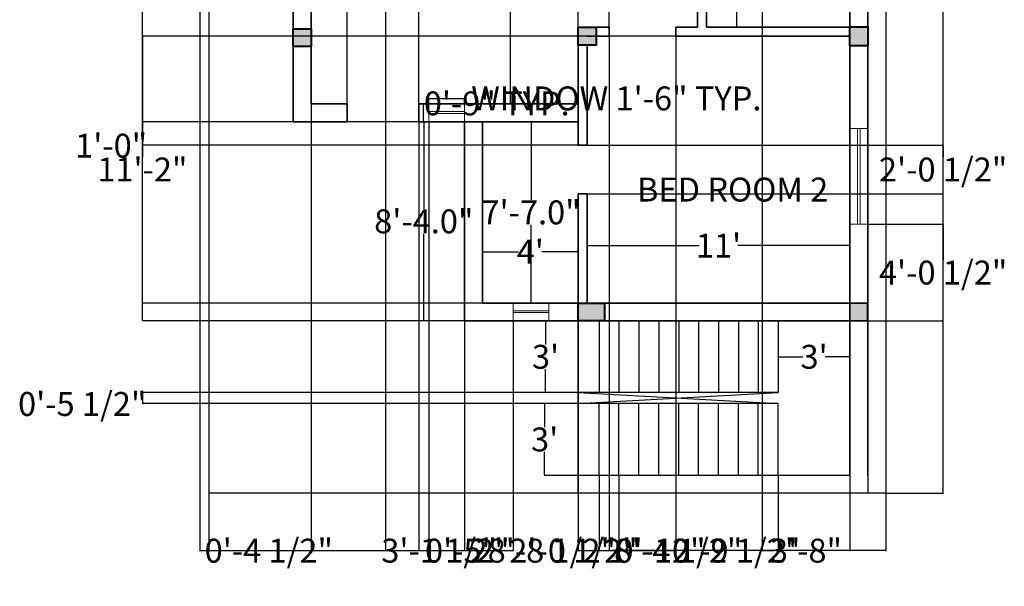
# Model space of a CAD drawing. Units: inches. Extents: x -132 to 363, y -548 to 79.
# Tile 1 of 3: x -132 to 363, y -548 to -264. Entities that reach past the tile are written whole.
import ezdxf

# ---------------------------------------------------------------- set-up
doc = ezdxf.new("R2010")
doc.units = ezdxf.units.IN
doc.header["$MEASUREMENT"] = 0
for name, color, linetype, lineweight in [('A-ANNO-DIMS', 2, 'Continuous', 18), ('A-AREA-IDEN', 7, 'Continuous', 25), ('A-COLS', 7, 'Continuous', 40), ('A-COLS-PATT', 252, 'Continuous', 13), ('A-FLOR-STRS', 3, 'Continuous', 25), ('A-GLAZ', 4, 'Continuous', 18), ('A-WALL', 7, 'Continuous', 35), ('C-PROP', 8, 'Continuous', 25)]:
    doc.layers.add(name, color=color, linetype=linetype, lineweight=lineweight)
doc.styles.get("Standard").update_dxf_attribs({"font": 'arial.ttf'})
doc.dimstyles.get("Standard").update_dxf_attribs({"dimtxt": 12, "dimasz": 0.18, "dimexe": 0.18, "dimexo": 0.0625, "dimgap": 0.09, "dimtad": 0, "dimtih": 1, "dimtoh": 1, "dimdec": 1, "dimzin": 0, "dimdsep": 46, "dimlunit": 3, "dimtxsty": 'Standard', "dimcen": 0.09, "dimadec": 0, "dimazin": 0, "dimtfac": 1, "dimtdec": 1, "dimtofl": 0, "dimtmove": 0, "dimatfit": 3, "dimfxl": 1, "dimtolj": 1, "dimtzin": 0, "dimarcsym": 0})

# ---------------------------------------------------------------- blocks, each defined once
blk = doc.blocks.new('*D6')
at = {"layer": 'A-ANNO-DIMS', "color": 0, "lineweight": -2, "transparency": 16777216}
for p, q in [((213.08, -219.61), (228.48, -219.61)), ((228.3, -219.79), (228.3, -237.52)), ((228.3, -267.43), (228.3, -249.7)), ((213.08, -267.61), (228.48, -267.61))]:
    blk.add_line(p, q, dxfattribs=at)
at = {"layer": 'A-ANNO-DIMS', "color": 0, "transparency": 16777216}
for points in [[(228.27, -219.79), (228.33, -219.79), (228.3, -219.61)], [(228.27, -267.43), (228.33, -267.43), (228.3, -267.61)]]:
    blk.add_solid(points, dxfattribs=at)
at = {"layer": 'Defpoints', "color": 0, "transparency": 16777216}
for p in [(213.02, -219.61), (213.02, -267.61), (228.3, -267.61)]:
    blk.add_point(p, dxfattribs=at)
at = {"layer": 'A-ANNO-DIMS', "color": 0, "transparency": 16777216, "insert": (228.3, -243.61), "char_height": 12, "attachment_point": 5}
blk.add_mtext("\\A1;4'", dxfattribs=at)
blk = doc.blocks.new('*D8')
at = {"layer": 'A-ANNO-DIMS', "color": 0, "lineweight": -2, "transparency": 16777216}
for p, q in [((153.02, -378.62), (153.02, -377.14)), ((153.2, -377.32), (209.31, -377.32)), ((284.84, -377.32), (228.72, -377.32)), ((285.02, -378.62), (285.02, -377.14))]:
    blk.add_line(p, q, dxfattribs=at)
at = {"layer": 'A-ANNO-DIMS', "color": 0, "transparency": 16777216}
for points in [[(153.2, -377.29), (153.2, -377.35), (153.02, -377.32)], [(284.84, -377.29), (284.84, -377.35), (285.02, -377.32)]]:
    blk.add_solid(points, dxfattribs=at)
at = {"layer": 'Defpoints', "color": 0, "transparency": 16777216}
for p in [(153.02, -378.68), (285.02, -377.32), (285.02, -378.68)]:
    blk.add_point(p, dxfattribs=at)
at = {"layer": 'A-ANNO-DIMS', "color": 0, "transparency": 16777216, "insert": (219.02, -377.32), "char_height": 12, "attachment_point": 5}
blk.add_mtext("\\A1;11'", dxfattribs=at)
blk = doc.blocks.new('*D9')
at = {"layer": 'A-ANNO-DIMS', "color": 0, "lineweight": -2, "transparency": 16777216}
for p, q in [((249.02, -433.05), (249.02, -432.93)), ((249.2, -433.11), (261.41, -433.11)), ((284.84, -433.11), (272.62, -433.11)), ((285.02, -433.05), (285.02, -432.93))]:
    blk.add_line(p, q, dxfattribs=at)
at = {"layer": 'A-ANNO-DIMS', "color": 0, "transparency": 16777216}
for points in [[(249.2, -433.08), (249.2, -433.14), (249.02, -433.11)], [(284.84, -433.08), (284.84, -433.14), (285.02, -433.11)]]:
    blk.add_solid(points, dxfattribs=at)
at = {"layer": 'Defpoints', "color": 0, "transparency": 16777216}
for p in [(249.02, -433.11), (285.02, -433.11), (285.02, -433.11)]:
    blk.add_point(p, dxfattribs=at)
at = {"layer": 'A-ANNO-DIMS', "color": 0, "transparency": 16777216, "insert": (267.02, -433.11), "char_height": 12, "attachment_point": 5}
blk.add_mtext("\\A1;3'", dxfattribs=at)
blk = doc.blocks.new('*D10')
at = {"layer": 'A-ANNO-DIMS', "color": 0, "lineweight": -2, "transparency": 16777216}
for p, q in [((148.45, -415.11), (132, -415.11)), ((132.18, -415.29), (132.18, -426.89)), ((132.18, -450.93), (132.18, -439.33)), ((148.45, -451.11), (132, -451.11))]:
    blk.add_line(p, q, dxfattribs=at)
at = {"layer": 'A-ANNO-DIMS', "color": 0, "transparency": 16777216}
for points in [[(132.15, -415.29), (132.21, -415.29), (132.18, -415.11)], [(132.15, -450.93), (132.21, -450.93), (132.18, -451.11)]]:
    blk.add_solid(points, dxfattribs=at)
at = {"layer": 'Defpoints', "color": 0, "transparency": 16777216}
for p in [(148.52, -415.11), (132.18, -451.11), (148.52, -451.11)]:
    blk.add_point(p, dxfattribs=at)
at = {"layer": 'A-ANNO-DIMS', "color": 0, "transparency": 16777216, "insert": (132.18, -433.11), "char_height": 12, "attachment_point": 5}
blk.add_mtext("\\A1;3'", dxfattribs=at)
blk = doc.blocks.new('*D11')
at = {"layer": 'A-ANNO-DIMS', "color": 0, "lineweight": -2, "transparency": 16777216}
for p, q in [((148.45, -456.61), (131.55, -456.61)), ((131.73, -456.79), (131.73, -468.39)), ((131.73, -492.43), (131.73, -480.83)), ((148.45, -492.61), (131.55, -492.61))]:
    blk.add_line(p, q, dxfattribs=at)
at = {"layer": 'A-ANNO-DIMS', "color": 0, "transparency": 16777216}
for points in [[(131.7, -456.79), (131.76, -456.79), (131.73, -456.61)], [(131.7, -492.43), (131.76, -492.43), (131.73, -492.61)]]:
    blk.add_solid(points, dxfattribs=at)
at = {"layer": 'Defpoints', "color": 0, "transparency": 16777216}
for p in [(148.52, -456.61), (131.73, -492.61), (148.52, -492.61)]:
    blk.add_point(p, dxfattribs=at)
at = {"layer": 'A-ANNO-DIMS', "color": 0, "transparency": 16777216, "insert": (131.73, -474.61), "char_height": 12, "attachment_point": 5}
blk.add_mtext("\\A1;3'", dxfattribs=at)
blk = doc.blocks.new('*D12')
at = {"layer": 'A-ANNO-DIMS', "color": 0, "lineweight": -2, "transparency": 16777216}
for p, q in [((100.52, -380.31), (100.52, -380.19)), ((100.7, -380.37), (118.66, -380.37)), ((148.34, -380.37), (130.37, -380.37)), ((148.52, -380.31), (148.52, -380.19))]:
    blk.add_line(p, q, dxfattribs=at)
at = {"layer": 'A-ANNO-DIMS', "color": 0, "transparency": 16777216}
for points in [[(100.7, -380.34), (100.7, -380.4), (100.52, -380.37)], [(148.34, -380.34), (148.34, -380.4), (148.52, -380.37)]]:
    blk.add_solid(points, dxfattribs=at)
at = {"layer": 'Defpoints', "color": 0, "transparency": 16777216}
for p in [(100.52, -380.37), (148.52, -380.37), (148.52, -380.37)]:
    blk.add_point(p, dxfattribs=at)
at = {"layer": 'A-ANNO-DIMS', "color": 0, "transparency": 16777216, "insert": (124.52, -380.37), "char_height": 12, "attachment_point": 5}
blk.add_mtext("\\A1;4'", dxfattribs=at)
blk = doc.blocks.new('*D13')
at = {"layer": 'A-ANNO-DIMS', "color": 0, "lineweight": -2, "transparency": 16777216}
for p, q in [((120.95, -315.11), (125.08, -315.11)), ((124.9, -315.29), (124.9, -354.39)), ((124.9, -405.93), (124.9, -366.82)), ((124.97, -406.11), (125.08, -406.11))]:
    blk.add_line(p, q, dxfattribs=at)
at = {"layer": 'A-ANNO-DIMS', "color": 0, "transparency": 16777216}
for points in [[(124.87, -315.29), (124.93, -315.29), (124.9, -315.11)], [(124.87, -405.93), (124.93, -405.93), (124.9, -406.11)]]:
    blk.add_solid(points, dxfattribs=at)
at = {"layer": 'Defpoints', "color": 0, "transparency": 16777216}
for p in [(120.89, -315.11), (124.9, -406.11), (124.9, -406.11)]:
    blk.add_point(p, dxfattribs=at)
at = {"layer": 'A-ANNO-DIMS', "color": 0, "transparency": 16777216, "insert": (124.9, -360.61), "char_height": 12, "attachment_point": 5}
blk.add_mtext('\\A1;7\'-7.0"', dxfattribs=at)
blk = doc.blocks.new('*D14')
at = {"layer": 'A-ANNO-DIMS', "color": 0, "lineweight": -2, "transparency": 16777216}
for p, q in [((91.45, -315.11), (70.85, -315.11)), ((71.03, -315.29), (71.03, -358.89)), ((71.03, -414.93), (71.03, -371.32)), ((91.45, -415.11), (70.85, -415.11))]:
    blk.add_line(p, q, dxfattribs=at)
at = {"layer": 'A-ANNO-DIMS', "color": 0, "transparency": 16777216}
for points in [[(71, -315.29), (71.06, -315.29), (71.03, -315.11)], [(71, -414.93), (71.06, -414.93), (71.03, -415.11)]]:
    blk.add_solid(points, dxfattribs=at)
at = {"layer": 'Defpoints', "color": 0, "transparency": 16777216}
for p in [(91.52, -315.11), (71.03, -415.11), (91.52, -415.11)]:
    blk.add_point(p, dxfattribs=at)
at = {"layer": 'A-ANNO-DIMS', "color": 0, "transparency": 16777216, "insert": (71.03, -365.11), "char_height": 12, "attachment_point": 5}
blk.add_mtext('\\A1;8\'-4.0"', dxfattribs=at)
blk = doc.blocks.new('*D16')
at = {"layer": 'A-ANNO-DIMS', "color": 0, "lineweight": -2, "transparency": 16777216}
for p, q in [((148.45, -92.11), (114.32, -92.11)), ((114.5, -92.29), (114.5, -192.89)), ((114.5, -305.93), (114.5, -205.32)), ((148.45, -306.11), (114.32, -306.11))]:
    blk.add_line(p, q, dxfattribs=at)
at = {"layer": 'A-ANNO-DIMS', "color": 0, "transparency": 16777216}
for points in [[(114.47, -92.29), (114.53, -92.29), (114.5, -92.11)], [(114.47, -305.93), (114.53, -305.93), (114.5, -306.11)]]:
    blk.add_solid(points, dxfattribs=at)
at = {"layer": 'Defpoints', "color": 0, "transparency": 16777216}
for p in [(148.52, -92.11), (114.5, -306.11), (148.52, -306.11)]:
    blk.add_point(p, dxfattribs=at)
at = {"layer": 'A-ANNO-DIMS', "color": 0, "transparency": 16777216, "insert": (114.5, -199.11), "char_height": 12, "attachment_point": 5}
blk.add_mtext('\\A1;17\'-10.0"', dxfattribs=at)
blk = doc.blocks.new('WIN-48IN')
for p, q in [((48, 9), (0, 9)), ((0, 9), (0, 0)), ((0, 5.12), (48, 5.12)), ((48, 5.12), (0, 5.12)), ((48, 0), (48, 9)), ((0, 3.8), (48, 3.8)), ((0, 0), (48, 0))]:
    blk.add_line(p, q)
blk = doc.blocks.new('WIN-18IN')
for p, q in [((18, 9), (0, 9)), ((0, 9), (0, 0)), ((0, 6), (0, 0)), ((18, 5.06), (0, 5.06)), ((18, 0), (18, 9)), ((18, 0), (18, 6)), ((18, 4.2), (0, 4.2)), ((0, 0), (18, 0)), ((0, 0), (18, 0)), ((0, 0), (18, 0))]:
    blk.add_line(p, q)
blk = doc.blocks.new('*D23')
at = {"layer": 'A-ANNO-DIMS', "color": 0, "lineweight": -2, "transparency": 16777216}
for p, q in [((73.52, -306.05), (73.52, -303.23)), ((73.7, -303.41), (91.34, -303.41)), ((91.52, -306.05), (91.52, -303.23)), ((91.52, -303.41), (91.7, -303.41))]:
    blk.add_line(p, q, dxfattribs=at)
at = {"layer": 'A-ANNO-DIMS', "color": 0, "transparency": 16777216}
for points in [[(73.7, -303.38), (73.7, -303.44), (73.52, -303.41)], [(91.34, -303.38), (91.34, -303.44), (91.52, -303.41)]]:
    blk.add_solid(points, dxfattribs=at)
at = {"layer": 'Defpoints', "color": 0, "transparency": 16777216}
for p in [(73.52, -306.11), (91.52, -303.41), (91.52, -306.11)]:
    blk.add_point(p, dxfattribs=at)
at = {"layer": 'A-ANNO-DIMS', "color": 0, "transparency": 16777216, "insert": (167.71, -303.41), "char_height": 12, "attachment_point": 5}
blk.add_mtext('\\A1;WINDOW 1\'-6" TYP.', dxfattribs=at)
blk = doc.blocks.new('*D24')
at = {"layer": 'A-ANNO-DIMS', "color": 0, "lineweight": -2, "transparency": 16777216}
for p, q in [((73.45, -306.11), (70.64, -306.11)), ((70.82, -306.11), (70.82, -305.93)), ((70.82, -305.93), (71, -305.93)), ((70.82, -314.93), (70.82, -306.29)), ((73.45, -315.11), (70.64, -315.11))]:
    blk.add_line(p, q, dxfattribs=at)
at = {"layer": 'A-ANNO-DIMS', "color": 0, "transparency": 16777216}
for points in [[(70.79, -306.29), (70.85, -306.29), (70.82, -306.11)], [(70.79, -314.93), (70.85, -314.93), (70.82, -315.11)]]:
    blk.add_solid(points, dxfattribs=at)
at = {"layer": 'Defpoints', "color": 0, "transparency": 16777216}
for p in [(70.82, -306.11), (73.52, -306.11), (73.52, -315.11)]:
    blk.add_point(p, dxfattribs=at)
at = {"layer": 'A-ANNO-DIMS', "color": 0, "transparency": 16777216, "insert": (107.66, -305.93), "char_height": 12, "attachment_point": 5}
blk.add_mtext('\\A1;0\'-9" TYP.', dxfattribs=at)
blk = doc.blocks.new('*D25')
at = {"layer": 'A-ANNO-DIMS', "color": 0, "lineweight": -2, "transparency": 16777216}
for p, q in [((-41.48, -501.67), (-41.48, -530.59)), ((303.02, -501.67), (303.02, -530.59)), ((-41.3, -530.41), (95.98, -530.41)), ((302.84, -530.41), (165.55, -530.41))]:
    blk.add_line(p, q, dxfattribs=at)
at = {"layer": 'A-ANNO-DIMS', "color": 0, "transparency": 16777216}
for points in [[(-41.3, -530.38), (-41.3, -530.44), (-41.48, -530.41)], [(302.84, -530.38), (302.84, -530.44), (303.02, -530.41)]]:
    blk.add_solid(points, dxfattribs=at)
at = {"layer": 'Defpoints', "color": 0, "transparency": 16777216}
for p in [(-41.48, -501.61), (303.02, -501.61), (303.02, -530.41)]:
    blk.add_point(p, dxfattribs=at)
at = {"layer": 'A-ANNO-DIMS', "color": 0, "transparency": 16777216, "insert": (130.77, -530.41), "char_height": 12, "attachment_point": 5}
blk.add_mtext('\\A1;28\'-8 1/2"', dxfattribs=at)
blk = doc.blocks.new('*D26')
at = {"layer": 'A-ANNO-DIMS', "color": 0, "lineweight": -2, "transparency": 16777216}
for p, q in [((303.08, 32.39), (332, 32.39)), ((331.82, 32.21), (331.82, -228.39)), ((331.82, -501.43), (331.82, -240.82)), ((303.08, -501.61), (332, -501.61))]:
    blk.add_line(p, q, dxfattribs=at)
at = {"layer": 'A-ANNO-DIMS', "color": 0, "transparency": 16777216}
for points in [[(331.79, 32.21), (331.85, 32.21), (331.82, 32.39)], [(331.79, -501.43), (331.85, -501.43), (331.82, -501.61)]]:
    blk.add_solid(points, dxfattribs=at)
at = {"layer": 'Defpoints', "color": 0, "transparency": 16777216}
for p in [(303.02, 32.39), (303.02, -501.61), (331.82, -501.61)]:
    blk.add_point(p, dxfattribs=at)
at = {"layer": 'A-ANNO-DIMS', "color": 0, "transparency": 16777216, "insert": (331.82, -234.61), "char_height": 12, "attachment_point": 5}
blk.add_mtext('\\A1;44\'-6"', dxfattribs=at)
blk = doc.blocks.new('*D29')
at = {"layer": 'A-ANNO-DIMS', "color": 0, "lineweight": -2, "transparency": 16777216}
for p, q in [((14.42, 14.33), (14.42, -530.59)), ((51.75, 14.33), (51.75, -530.59)), ((14.6, -530.41), (51.57, -530.41)), ((51.75, -530.41), (51.93, -530.41))]:
    blk.add_line(p, q, dxfattribs=at)
at = {"layer": 'A-ANNO-DIMS', "color": 0, "transparency": 16777216}
for points in [[(14.6, -530.38), (14.6, -530.44), (14.42, -530.41)], [(51.57, -530.38), (51.57, -530.44), (51.75, -530.41)]]:
    blk.add_solid(points, dxfattribs=at)
at = {"layer": 'Defpoints', "color": 0, "transparency": 16777216}
for p in [(14.42, 14.39), (51.75, 14.39), (51.75, -530.41)]:
    blk.add_point(p, dxfattribs=at)
at = {"layer": 'A-ANNO-DIMS', "color": 0, "transparency": 16777216, "insert": (81.94, -530.41), "char_height": 12, "attachment_point": 5}
blk.add_mtext('\\A1;3\'-1 1/2"', dxfattribs=at)
blk = doc.blocks.new('*D30')
at = {"layer": 'A-ANNO-DIMS', "color": 0, "lineweight": -2, "transparency": 16777216}
for p, q in [((240.9, 14.33), (240.9, -530.59)), ((285.02, 14.33), (285.02, -530.59)), ((241.08, -530.41), (246.92, -530.41)), ((284.84, -530.41), (278.99, -530.41))]:
    blk.add_line(p, q, dxfattribs=at)
at = {"layer": 'A-ANNO-DIMS', "color": 0, "transparency": 16777216}
for points in [[(241.08, -530.38), (241.08, -530.44), (240.9, -530.41)], [(284.84, -530.38), (284.84, -530.44), (285.02, -530.41)]]:
    blk.add_solid(points, dxfattribs=at)
at = {"layer": 'Defpoints', "color": 0, "transparency": 16777216}
for p in [(240.9, 14.39), (285.02, 14.39), (285.02, -530.41)]:
    blk.add_point(p, dxfattribs=at)
at = {"layer": 'A-ANNO-DIMS', "color": 0, "transparency": 16777216, "insert": (262.96, -530.41), "char_height": 12, "attachment_point": 5}
blk.add_mtext('\\A1;3\'-8"', dxfattribs=at)
blk = doc.blocks.new('*D37')
at = {"layer": 'A-ANNO-DIMS', "color": 0, "lineweight": -2, "transparency": 16777216}
for p, q in [((294.08, -366.55), (332, -366.55)), ((331.82, -366.73), (331.82, -384.53)), ((331.82, -414.93), (331.82, -397.12)), ((294.08, -415.11), (332, -415.11))]:
    blk.add_line(p, q, dxfattribs=at)
at = {"layer": 'A-ANNO-DIMS', "color": 0, "transparency": 16777216}
for points in [[(331.79, -366.73), (331.85, -366.73), (331.82, -366.55)], [(331.79, -414.93), (331.85, -414.93), (331.82, -415.11)]]:
    blk.add_solid(points, dxfattribs=at)
at = {"layer": 'Defpoints', "color": 0, "transparency": 16777216}
for p in [(294.02, -366.55), (294.02, -415.11), (331.82, -415.11)]:
    blk.add_point(p, dxfattribs=at)
at = {"layer": 'A-ANNO-DIMS', "color": 0, "transparency": 16777216, "insert": (331.82, -390.83), "char_height": 12, "attachment_point": 5}
blk.add_mtext('\\A1;4\'-0 1/2"', dxfattribs=at)
blk = doc.blocks.new('*D38')
at = {"layer": 'A-ANNO-DIMS', "color": 0, "lineweight": -2, "transparency": 16777216}
for p, q in [((284.95, -272.11), (-70.46, -272.11)), ((-70.28, -272.29), (-70.28, -332.99)), ((-70.28, -405.93), (-70.28, -345.22)), ((293.95, -406.11), (-70.46, -406.11))]:
    blk.add_line(p, q, dxfattribs=at)
at = {"layer": 'A-ANNO-DIMS', "color": 0, "transparency": 16777216}
for points in [[(-70.31, -272.29), (-70.25, -272.29), (-70.28, -272.11)], [(-70.31, -405.93), (-70.25, -405.93), (-70.28, -406.11)]]:
    blk.add_solid(points, dxfattribs=at)
at = {"layer": 'Defpoints', "color": 0, "transparency": 16777216}
for p in [(285.02, -272.11), (-70.28, -406.11), (294.02, -406.11)]:
    blk.add_point(p, dxfattribs=at)
at = {"layer": 'A-ANNO-DIMS', "color": 0, "transparency": 16777216, "insert": (-70.28, -339.11), "char_height": 12, "attachment_point": 5}
blk.add_mtext('\\A1;11\'-2"', dxfattribs=at)
blk = doc.blocks.new('*D39')
at = {"layer": 'A-ANNO-DIMS', "color": 0, "lineweight": -2, "transparency": 16777216}
for p, q in [((32.59, -306.05), (32.59, 61.37)), ((32.77, 61.19), (34.56, 61.19)), ((68.41, 61.19), (66.63, 61.19)), ((68.59, -306.05), (68.59, 61.37))]:
    blk.add_line(p, q, dxfattribs=at)
at = {"layer": 'A-ANNO-DIMS', "color": 0, "transparency": 16777216}
for points in [[(32.77, 61.22), (32.77, 61.16), (32.59, 61.19)], [(68.41, 61.22), (68.41, 61.16), (68.59, 61.19)]]:
    blk.add_solid(points, dxfattribs=at)
at = {"layer": 'Defpoints', "color": 0, "transparency": 16777216}
for p in [(68.59, 61.19), (32.59, -306.11), (68.59, -306.11)]:
    blk.add_point(p, dxfattribs=at)
at = {"layer": 'A-ANNO-DIMS', "color": 0, "transparency": 16777216, "insert": (50.59, 61.19), "char_height": 12, "attachment_point": 5}
blk.add_mtext('\\A1;3\'-0"', dxfattribs=at)
blk = doc.blocks.new('*D40')
at = {"layer": 'A-ANNO-DIMS', "color": 0, "lineweight": -2, "transparency": 16777216}
for p, q in [((14.42, -306.05), (14.42, 61.37)), ((14.6, 61.19), (32.41, 61.19)), ((32.59, -306.05), (32.59, 61.37)), ((32.59, 61.19), (32.77, 61.19))]:
    blk.add_line(p, q, dxfattribs=at)
at = {"layer": 'A-ANNO-DIMS', "color": 0, "transparency": 16777216}
for points in [[(14.6, 61.22), (14.6, 61.16), (14.42, 61.19)], [(32.41, 61.22), (32.41, 61.16), (32.59, 61.19)]]:
    blk.add_solid(points, dxfattribs=at)
at = {"layer": 'Defpoints', "color": 0, "transparency": 16777216}
for p in [(32.59, 61.19), (14.42, -306.11), (32.59, -306.11)]:
    blk.add_point(p, dxfattribs=at)
at = {"layer": 'A-ANNO-DIMS', "color": 0, "transparency": 16777216, "insert": (48.25, 61.19), "char_height": 12, "attachment_point": 5}
blk.add_mtext('\\A1;1\'-6"', dxfattribs=at)
blk = doc.blocks.new('*D41')
at = {"layer": 'A-ANNO-DIMS', "color": 0, "lineweight": -2, "transparency": 16777216}
for p, q in [((68.59, -315.17), (68.59, -530.59)), ((73.52, -315.17), (73.52, -530.59)), ((68.77, -530.41), (73.34, -530.41)), ((73.52, -530.41), (73.7, -530.41))]:
    blk.add_line(p, q, dxfattribs=at)
at = {"layer": 'A-ANNO-DIMS', "color": 0, "transparency": 16777216}
for points in [[(68.77, -530.38), (68.77, -530.44), (68.59, -530.41)], [(73.34, -530.38), (73.34, -530.44), (73.52, -530.41)]]:
    blk.add_solid(points, dxfattribs=at)
at = {"layer": 'Defpoints', "color": 0, "transparency": 16777216}
for p in [(68.59, -315.11), (73.52, -315.11), (73.52, -530.41)]:
    blk.add_point(p, dxfattribs=at)
at = {"layer": 'A-ANNO-DIMS', "color": 0, "transparency": 16777216, "insert": (89.74, -530.41), "char_height": 12, "attachment_point": 5}
blk.add_mtext('\\A1;0\'-5"', dxfattribs=at)
blk = doc.blocks.new('*D42')
at = {"layer": 'A-ANNO-DIMS', "color": 0, "lineweight": -2, "transparency": 16777216}
for p, q in [((91.52, -415.17), (91.52, -530.59)), ((115.9, -415.17), (115.9, -530.59)), ((91.7, -530.41), (115.72, -530.41)), ((115.9, -530.41), (116.08, -530.41))]:
    blk.add_line(p, q, dxfattribs=at)
at = {"layer": 'A-ANNO-DIMS', "color": 0, "transparency": 16777216}
for points in [[(91.7, -530.38), (91.7, -530.44), (91.52, -530.41)], [(115.72, -530.38), (115.72, -530.44), (115.9, -530.41)]]:
    blk.add_solid(points, dxfattribs=at)
at = {"layer": 'Defpoints', "color": 0, "transparency": 16777216}
for p in [(91.52, -415.11), (115.9, -415.11), (115.9, -530.41)]:
    blk.add_point(p, dxfattribs=at)
at = {"layer": 'A-ANNO-DIMS', "color": 0, "transparency": 16777216, "insert": (146.21, -530.41), "char_height": 12, "attachment_point": 5}
blk.add_mtext('\\A1;2\'-0 1/2"', dxfattribs=at)
blk = doc.blocks.new('*D43')
at = {"layer": 'A-ANNO-DIMS', "color": 0, "lineweight": -2, "transparency": 16777216}
for p, q in [((148.52, -492.67), (148.52, -530.59)), ((249.02, -492.67), (249.02, -530.59)), ((148.7, -530.41), (168.74, -530.41)), ((248.84, -530.41), (228.79, -530.41))]:
    blk.add_line(p, q, dxfattribs=at)
at = {"layer": 'A-ANNO-DIMS', "color": 0, "transparency": 16777216}
for points in [[(148.7, -530.38), (148.7, -530.44), (148.52, -530.41)], [(248.84, -530.38), (248.84, -530.44), (249.02, -530.41)]]:
    blk.add_solid(points, dxfattribs=at)
at = {"layer": 'Defpoints', "color": 0, "transparency": 16777216}
for p in [(148.52, -492.61), (249.02, -492.61), (249.02, -530.41)]:
    blk.add_point(p, dxfattribs=at)
at = {"layer": 'A-ANNO-DIMS', "color": 0, "transparency": 16777216, "insert": (198.77, -530.41), "char_height": 12, "attachment_point": 5}
blk.add_mtext('\\A1;8\'-4 1/2"', dxfattribs=at)
blk = doc.blocks.new('*D45')
at = {"layer": 'A-ANNO-DIMS', "color": 0, "lineweight": -2, "transparency": 16777216}
for p, q in [((164.09, -272.17), (164.09, -530.59)), ((197.59, -272.17), (197.59, -530.59)), ((164.27, -530.41), (197.41, -530.41)), ((197.59, -530.41), (197.77, -530.41))]:
    blk.add_line(p, q, dxfattribs=at)
at = {"layer": 'A-ANNO-DIMS', "color": 0, "transparency": 16777216}
for points in [[(164.27, -530.38), (164.27, -530.44), (164.09, -530.41)], [(197.41, -530.38), (197.41, -530.44), (197.59, -530.41)]]:
    blk.add_solid(points, dxfattribs=at)
at = {"layer": 'Defpoints', "color": 0, "transparency": 16777216}
for p in [(164.09, -272.11), (197.59, -272.11), (197.59, -530.41)]:
    blk.add_point(p, dxfattribs=at)
at = {"layer": 'A-ANNO-DIMS', "color": 0, "transparency": 16777216, "insert": (227.89, -530.41), "char_height": 12, "attachment_point": 5}
blk.add_mtext('\\A1;2\'-9 1/2"', dxfattribs=at)
blk = doc.blocks.new('*D47')
at = {"layer": 'A-ANNO-DIMS', "color": 0, "lineweight": -2, "transparency": 16777216}
for p, q in [((153.08, -326.96), (332, -326.96)), ((331.82, -327.14), (331.82, -332.81)), ((331.82, -351.07), (331.82, -345.4)), ((153.08, -351.25), (332, -351.25))]:
    blk.add_line(p, q, dxfattribs=at)
at = {"layer": 'A-ANNO-DIMS', "color": 0, "transparency": 16777216}
for points in [[(331.79, -327.14), (331.85, -327.14), (331.82, -326.96)], [(331.79, -351.07), (331.85, -351.07), (331.82, -351.25)]]:
    blk.add_solid(points, dxfattribs=at)
at = {"layer": 'Defpoints', "color": 0, "transparency": 16777216}
for p in [(153.02, -326.96), (153.02, -351.25), (331.82, -351.25)]:
    blk.add_point(p, dxfattribs=at)
at = {"layer": 'A-ANNO-DIMS', "color": 0, "transparency": 16777216, "insert": (331.82, -339.11), "char_height": 12, "attachment_point": 5}
blk.add_mtext('\\A1;2\'-0 1/2"', dxfattribs=at)
blk = doc.blocks.new('*D49')
at = {"layer": 'A-ANNO-DIMS', "color": 0, "lineweight": -2, "transparency": 16777216}
for p, q in [((148.45, -315.11), (-70.46, -315.11)), ((-70.28, -315.29), (-70.28, -326.78)), ((148.45, -326.96), (-70.46, -326.96)), ((-70.28, -327.14), (-70.46, -327.14)), ((-70.28, -326.96), (-70.28, -327.14))]:
    blk.add_line(p, q, dxfattribs=at)
at = {"layer": 'A-ANNO-DIMS', "color": 0, "transparency": 16777216}
for points in [[(-70.31, -315.29), (-70.25, -315.29), (-70.28, -315.11)], [(-70.31, -326.78), (-70.25, -326.78), (-70.28, -326.96)]]:
    blk.add_solid(points, dxfattribs=at)
at = {"layer": 'Defpoints', "color": 0, "transparency": 16777216}
for p in [(148.52, -315.11), (-70.28, -326.96), (148.52, -326.96)]:
    blk.add_point(p, dxfattribs=at)
at = {"layer": 'A-ANNO-DIMS', "color": 0, "transparency": 16777216, "insert": (-85.94, -327.14), "char_height": 12, "attachment_point": 5}
blk.add_mtext('\\A1;1\'-0"', dxfattribs=at)
blk = doc.blocks.new('*D51')
at = {"layer": 'A-ANNO-DIMS', "color": 0, "lineweight": -2, "transparency": 16777216}
for p, q in [((159.02, -492.67), (159.02, -530.59)), ((169.02, -492.67), (169.02, -530.59)), ((159.2, -530.41), (168.84, -530.41)), ((169.02, -530.41), (169.2, -530.41))]:
    blk.add_line(p, q, dxfattribs=at)
at = {"layer": 'A-ANNO-DIMS', "color": 0, "transparency": 16777216}
for points in [[(159.2, -530.38), (159.2, -530.44), (159.02, -530.41)], [(168.84, -530.38), (168.84, -530.44), (169.02, -530.41)]]:
    blk.add_solid(points, dxfattribs=at)
at = {"layer": 'Defpoints', "color": 0, "transparency": 16777216}
for p in [(159.02, -492.61), (169.02, -492.61), (169.02, -530.41)]:
    blk.add_point(p, dxfattribs=at)
at = {"layer": 'A-ANNO-DIMS', "color": 0, "transparency": 16777216, "insert": (189.9, -530.41), "char_height": 12, "attachment_point": 5}
blk.add_mtext('\\A1;0\'-10"', dxfattribs=at)
blk = doc.blocks.new('*D53')
at = {"layer": 'A-ANNO-DIMS', "color": 0, "lineweight": -2, "transparency": 16777216}
for p, q in [((5.35, 23.39), (-70.46, 23.39)), ((-70.28, 23.21), (-70.28, -189.56)), ((-70.28, -414.93), (-70.28, -202.16)), ((91.45, -415.11), (-70.46, -415.11))]:
    blk.add_line(p, q, dxfattribs=at)
at = {"layer": 'A-ANNO-DIMS', "color": 0, "transparency": 16777216}
for points in [[(-70.31, 23.21), (-70.25, 23.21), (-70.28, 23.39)], [(-70.31, -414.93), (-70.25, -414.93), (-70.28, -415.11)]]:
    blk.add_solid(points, dxfattribs=at)
at = {"layer": 'Defpoints', "color": 0, "transparency": 16777216}
for p in [(5.42, 23.39), (-70.28, -415.11), (91.52, -415.11)]:
    blk.add_point(p, dxfattribs=at)
at = {"layer": 'A-ANNO-DIMS', "color": 0, "transparency": 16777216, "insert": (-70.28, -195.86), "char_height": 12, "attachment_point": 5}
blk.add_mtext('\\A1;36\'-6 1/2"', dxfattribs=at)
blk = doc.blocks.new('*D55')
at = {"layer": 'A-ANNO-DIMS', "color": 0, "lineweight": -2, "transparency": 16777216}
for p, q in [((-41.48, -501.67), (-41.48, -530.59)), ((-36.98, -501.67), (-36.98, -530.59)), ((-41.3, -530.41), (-37.16, -530.41)), ((-36.98, -530.41), (-36.8, -530.41))]:
    blk.add_line(p, q, dxfattribs=at)
at = {"layer": 'A-ANNO-DIMS', "color": 0, "transparency": 16777216}
for points in [[(-41.3, -530.38), (-41.3, -530.44), (-41.48, -530.41)], [(-37.16, -530.38), (-37.16, -530.44), (-36.98, -530.41)]]:
    blk.add_solid(points, dxfattribs=at)
at = {"layer": 'Defpoints', "color": 0, "transparency": 16777216}
for p in [(-41.48, -501.61), (-36.98, -501.61), (-36.98, -530.41)]:
    blk.add_point(p, dxfattribs=at)
at = {"layer": 'A-ANNO-DIMS', "color": 0, "transparency": 16777216, "insert": (-6.78, -530.41), "char_height": 12, "attachment_point": 5}
blk.add_mtext('\\A1;0\'-4 1/2"', dxfattribs=at)
blk = doc.blocks.new('*D56')
at = {"layer": 'A-ANNO-DIMS', "color": 0, "lineweight": -2, "transparency": 16777216}
for p, q in [((148.45, -451.11), (-70.46, -451.11)), ((-70.28, -451.29), (-70.28, -456.43)), ((148.45, -456.61), (-70.46, -456.61)), ((-70.28, -456.79), (-70.46, -456.79)), ((-70.28, -456.61), (-70.28, -456.79))]:
    blk.add_line(p, q, dxfattribs=at)
at = {"layer": 'A-ANNO-DIMS', "color": 0, "transparency": 16777216}
for points in [[(-70.31, -451.29), (-70.25, -451.29), (-70.28, -451.11)], [(-70.31, -456.43), (-70.25, -456.43), (-70.28, -456.61)]]:
    blk.add_solid(points, dxfattribs=at)
at = {"layer": 'Defpoints', "color": 0, "transparency": 16777216}
for p in [(148.52, -451.11), (-70.28, -456.61), (148.52, -456.61)]:
    blk.add_point(p, dxfattribs=at)
at = {"layer": 'A-ANNO-DIMS', "color": 0, "transparency": 16777216, "insert": (-100.48, -456.79), "char_height": 12, "attachment_point": 5}
blk.add_mtext('\\A1;0\'-5 1/2"', dxfattribs=at)
blk = doc.blocks.new('*D57')
at = {"layer": 'A-ANNO-DIMS', "color": 0, "lineweight": -2, "transparency": 16777216}
for p, q in [((148.52, -267.55), (148.52, 61.37)), ((148.7, 61.19), (163.91, 61.19)), ((164.09, -267.55), (164.09, 61.37)), ((164.09, 61.19), (164.27, 61.19))]:
    blk.add_line(p, q, dxfattribs=at)
at = {"layer": 'A-ANNO-DIMS', "color": 0, "transparency": 16777216}
for points in [[(148.7, 61.22), (148.7, 61.16), (148.52, 61.19)], [(163.91, 61.22), (163.91, 61.16), (164.09, 61.19)]]:
    blk.add_solid(points, dxfattribs=at)
at = {"layer": 'Defpoints', "color": 0, "transparency": 16777216}
for p in [(164.09, 61.19), (148.52, -267.61), (164.09, -267.61)]:
    blk.add_point(p, dxfattribs=at)
at = {"layer": 'A-ANNO-DIMS', "color": 0, "transparency": 16777216, "insert": (193.73, 61.19), "char_height": 12, "attachment_point": 5}
blk.add_mtext('\\A1;1\'-3 1/2"', dxfattribs=at)

msp = doc.modelspace()

# ---------------------------------------------------------------- hatches: boundary and pattern name
at = {"layer": 'A-COLS-PATT'}
h = msp.add_hatch(color=256, dxfattribs=at)
h.dxf.hatch_style = 1
h.paths.add_polyline_path([(14.42, 23.39), (6.02, 23.39), (5.42, 23.39), (5.42, 14.39), (14.42, 14.39)])
h.paths.add_polyline_path([(14.42, -87.61), (5.42, -87.61), (5.42, -96.61), (14.42, -96.61)])
h.paths.add_polyline_path([(153.02, -87.61), (148.56, -87.61), (148.56, -96.61), (153.02, -96.61)])
h.paths.add_polyline_path([(157.56, -87.61), (153.02, -87.61), (153.02, -92.11), (157.56, -92.11)])
h.paths.add_polyline_path([(157.56, -92.11), (153.02, -92.11), (153.02, -96.61), (157.56, -96.61)])
h.paths.add_polyline_path([(294.02, -87.49), (285.02, -87.49), (285.02, -96.49), (294.02, -96.49)])
h.paths.add_polyline_path([(294.02, -215.01), (285.02, -215.01), (285.02, -224.01), (294.02, -224.01)])
h.paths.add_polyline_path([(294.02, -267.43), (285.02, -267.43), (285.02, -277.01), (294.02, -277.01)])
h.paths.add_polyline_path([(294.02, -406.11), (285.02, -406.11), (285.02, -415.11), (294.02, -415.11)])
h.paths.add_polyline_path([(161.71, -406.11), (148.52, -406.11), (148.52, -415.11), (161.71, -415.11)])
h.paths.add_polyline_path([(157.51, -267.61), (148.52, -267.61), (148.52, -276.61), (157.51, -276.61)])
h.paths.add_polyline_path([(14.42, -268.43), (5.42, -268.43), (5.42, -277.43), (14.42, -277.43)])

# ---------------------------------------------------------------- linework, layer by layer
at = {"layer": 'A-COLS'}
msp.add_line((294.02, -415.11), (294.02, -406.11), dxfattribs=at)
for points in [[(5.42, -268.43), (14.42, -268.43), (14.42, -277.43), (5.42, -277.43)], [(148.51, -267.61), (157.51, -267.61), (157.51, -276.61), (148.51, -276.61)], [(285.02, -267.43), (294.02, -267.43), (294.02, -277.01), (285.02, -277.01)], [(148.52, -406.11), (161.71, -406.11), (161.71, -415.11), (148.52, -415.11)]]:
    msp.add_lwpolyline(points, close=True, dxfattribs=at)
at = {"layer": 'A-FLOR-STRS'}
for p, q in [((159.02, -415.11), (159.02, -451.11)), ((169.02, -415.11), (169.02, -451.11)), ((179.02, -415.11), (179.02, -451.11)), ((189.02, -415.11), (189.02, -451.11)), ((199.02, -415.11), (199.02, -451.11)), ((209.02, -415.11), (209.02, -451.11)), ((219.02, -415.11), (219.02, -451.11)), ((229.02, -415.11), (229.02, -451.11)), ((239.02, -415.11), (239.02, -451.11)), ((285.02, -415.11), (249.02, -415.11)), ((249.02, -415.11), (249.02, -451.11)), ((249.02, -451.11), (148.52, -451.11)), ((148.52, -451.11), (249.02, -456.61)), ((148.52, -456.61), (249.02, -451.11)), ((249.02, -456.61), (148.52, -456.61)), ((159.02, -492.61), (159.02, -456.61)), ((169.02, -492.61), (169.02, -456.61)), ((179.02, -492.61), (179.02, -456.61)), ((189.02, -492.61), (189.02, -456.61)), ((199.02, -492.61), (199.02, -456.61)), ((209.02, -492.61), (209.02, -456.61)), ((219.02, -492.61), (219.02, -456.61)), ((229.02, -492.61), (229.02, -456.61)), ((239.02, -492.61), (239.02, -456.61)), ((249.02, -492.61), (249.02, -456.61)), ((285.02, -492.61), (148.52, -492.61)), ((285.02, -492.61), (249.02, -492.61))]:
    msp.add_line(p, q, dxfattribs=at)
at = {"layer": 'A-WALL'}
for p, q in [((294.02, 23.39), (294.02, -492.61)), ((285.02, 14.39), (285.02, -492.61)), ((5.42, -40.26), (5.42, -315.11)), ((14.42, -40.26), (14.42, -306.11)), ((208.52, -254.12), (208.52, -267.61)), ((213.02, -254.12), (213.02, -267.61)), ((157.51, -267.61), (148.52, -267.61)), ((148.52, -267.61), (148.52, -326.96)), ((157.51, -272.11), (157.51, -267.61)), ((157.51, -267.61), (157.51, -272.11)), ((157.51, -267.61), (164.09, -267.61)), ((164.09, -267.61), (164.09, -272.11)), ((197.59, -267.61), (208.52, -267.61)), ((197.59, -267.61), (197.59, -272.11)), ((213.02, -267.61), (285.02, -267.61)), ((157.51, -272.11), (153.02, -272.11)), ((153.02, -276.61), (153.02, -326.96)), ((164.09, -272.11), (157.51, -272.11)), ((197.59, -272.11), (285.02, -272.11)), ((14.42, -306.11), (32.59, -306.11)), ((32.59, -315.11), (32.59, -306.11)), ((68.59, -306.11), (68.59, -315.11)), ((68.59, -306.11), (148.52, -306.11)), ((5.42, -315.11), (32.59, -315.11)), ((68.59, -315.11), (148.52, -315.11)), ((91.52, -315.11), (91.52, -415.11)), ((100.52, -315.11), (100.52, -406.11)), ((148.52, -326.96), (153.02, -326.96)), ((148.52, -351.25), (153.02, -351.25)), ((148.52, -351.25), (148.52, -501.61)), ((153.02, -351.25), (153.02, -406.11)), ((100.52, -406.11), (148.52, -406.11)), ((294.02, -406.11), (157.52, -406.11)), ((294.02, -407.11), (294.02, -416.11)), ((91.52, -415.11), (148.52, -415.11)), ((157.52, -415.11), (294.02, -415.11))]:
    msp.add_line(p, q, dxfattribs=at)
at = {"layer": 'C-PROP'}
for p, q in [((303.02, 32.39), (303.02, -501.61)), ((-41.48, 23.39), (-41.48, -501.61)), ((-36.98, 23.39), (-36.98, -501.61)), ((294.02, -492.61), (294.02, -501.61)), ((285.02, -501.61), (-36.98, -501.61)), ((303.02, -501.61), (285.02, -501.61))]:
    msp.add_line(p, q, dxfattribs=at)

# ---------------------------------------------------------------- block references
at = {"layer": 'A-GLAZ'}
for p in [(73.52, -315.11), (115.9, -415.11)]:
    msp.add_blockref('WIN-18IN', p, dxfattribs=at)
at = {"layer": 'A-GLAZ', "rotation": 269.9999999999999}
msp.add_blockref('WIN-48IN', (285.02, -318.55), dxfattribs=at)

# ---------------------------------------------------------------- texts
at = {"layer": 'A-AREA-IDEN'}
msp.add_text('BED ROOM 2', height=12, dxfattribs=at).set_placement((178.08, -355.17))

# ---------------------------------------------------------------- dimensions: what is measured, and where the dimension line sits
at = {"layer": 'A-ANNO-DIMS'}
for base, p1, p2, override, picture, middle in [((164.09, 61.19), (148.52, -267.61), (164.09, -267.61), {"dimdec": 1, "dimlfac": 1, "dimrnd": 0, "dimzin": 1, "dimdsep": 46, "dimlunit": 4, "dimfrac": 2}, '*D57', (193.73, 61.19)), ((32.59, 61.19), (14.42, -306.11), (32.59, -306.11), {"dimdec": 1, "dimlfac": 1, "dimrnd": 0, "dimzin": 1, "dimdsep": 46, "dimlunit": 4, "dimfrac": 2}, '*D40', (48.25, 61.19)), ((68.59, 61.19), (32.59, -306.11), (68.59, -306.11), {"dimdec": 1, "dimlfac": 1, "dimrnd": 0, "dimzin": 1, "dimdsep": 46, "dimlunit": 4, "dimfrac": 2}, '*D39', (50.59, 61.19)), ((51.75, -530.41), (14.42, 14.39), (51.75, 14.39), {"dimdec": 1, "dimlfac": 1, "dimrnd": 0, "dimzin": 1, "dimdsep": 46, "dimlunit": 4, "dimfrac": 2}, '*D29', (81.94, -530.41)), ((285.02, -530.41), (240.9, 14.39), (285.02, 14.39), {"dimdec": 1, "dimlfac": 1, "dimrnd": 0, "dimzin": 1, "dimdsep": 46, "dimlunit": 4, "dimfrac": 2}, '*D30', (262.96, -530.41)), ((197.59, -530.41), (164.09, -272.11), (197.59, -272.11), {"dimdec": 1, "dimlfac": 1, "dimrnd": 0, "dimzin": 1, "dimdsep": 46, "dimlunit": 4, "dimfrac": 2}, '*D45', (227.89, -530.41)), ((73.52, -530.41), (68.59, -315.11), (73.52, -315.11), {"dimdec": 1, "dimlfac": 1, "dimrnd": 0, "dimzin": 1, "dimdsep": 46, "dimlunit": 4, "dimfrac": 2}, '*D41', (89.74, -530.41)), ((285.02, -377.32), (153.02, -378.68), (285.02, -378.68), {"dimclrd": 0, "dimclre": 0, "dimclrt": 0}, '*D8', (219.02, -377.32)), ((148.52, -380.37), (100.52, -380.37), (148.52, -380.37), {"dimclrd": 0, "dimclre": 0, "dimclrt": 0}, '*D12', (124.52, -380.37)), ((115.9, -530.41), (91.52, -415.11), (115.9, -415.11), {"dimdec": 1, "dimlfac": 1, "dimrnd": 0, "dimzin": 1, "dimdsep": 46, "dimlunit": 4, "dimfrac": 2}, '*D42', (146.21, -530.41)), ((285.02, -433.11), (249.02, -433.11), (285.02, -433.11), {"dimclrd": 0, "dimclre": 0, "dimclrt": 0}, '*D9', (267.02, -433.11)), ((249.02, -530.41), (148.52, -492.61), (249.02, -492.61), {"dimdec": 1, "dimlfac": 1, "dimrnd": 0, "dimzin": 1, "dimdsep": 46, "dimlunit": 4, "dimfrac": 2}, '*D43', (198.77, -530.41)), ((169.02, -530.41), (159.02, -492.61), (169.02, -492.61), {"dimdec": 1, "dimlfac": 1, "dimrnd": 0, "dimzin": 1, "dimdsep": 46, "dimlunit": 4, "dimfrac": 2}, '*D51', (189.9, -530.41)), ((303.02, -530.41), (-41.48, -501.61), (303.02, -501.61), {"dimdec": 1, "dimlfac": 1, "dimrnd": 0, "dimzin": 1, "dimdsep": 46, "dimlunit": 4, "dimfrac": 2}, '*D25', (130.77, -530.41)), ((-36.98, -530.41), (-41.48, -501.61), (-36.98, -501.61), {"dimdec": 1, "dimlfac": 1, "dimrnd": 0, "dimzin": 1, "dimdsep": 46, "dimlunit": 4, "dimfrac": 2}, '*D55', (-6.78, -530.41))]:
    dim = msp.add_linear_dim(base=base, p1=p1, p2=p2, dimstyle='Standard', override=override, dxfattribs=at)
    dim.commit()
    dim.dimension.update_dxf_attribs({"geometry": picture, "text_midpoint": middle})
for base, p1, p2, override, picture, middle in [((331.82, -501.61), (303.02, 32.39), (303.02, -501.61), {"dimdec": 1, "dimlfac": 1, "dimrnd": 0, "dimzin": 1, "dimdsep": 46, "dimlunit": 4, "dimfrac": 2}, '*D26', (331.82, -234.61)), ((-70.28, -415.11), (5.42, 23.39), (91.52, -415.11), {"dimdec": 1, "dimlfac": 1, "dimrnd": 0, "dimzin": 1, "dimdsep": 46, "dimlunit": 4, "dimfrac": 2}, '*D53', (-70.28, -195.86)), ((114.5, -306.11), (148.52, -92.11), (148.52, -306.11), {"dimclrd": 0, "dimclre": 0, "dimclrt": 0}, '*D16', (114.5, -199.11)), ((228.3, -267.61), (213.02, -219.61), (213.02, -267.61), {"dimclrd": 0, "dimclre": 0, "dimclrt": 0}, '*D6', (228.3, -243.61)), ((-70.28, -406.11), (285.02, -272.11), (294.02, -406.11), {"dimdec": 1, "dimlfac": 1, "dimrnd": 0, "dimzin": 1, "dimdsep": 46, "dimlunit": 4, "dimfrac": 2}, '*D38', (-70.28, -339.11)), ((-70.2842, -326.9609), (148.5158, -315.108), (148.5158, -326.9609), {"dimdec": 1, "dimlfac": 1, "dimrnd": 0, "dimzin": 1, "dimdsep": 46, "dimlunit": 4, "dimfrac": 2}, '*D49', (-85.939, -327.1409)), ((71.03, -415.11), (91.52, -315.11), (91.52, -415.11), {"dimclrd": 0, "dimclre": 0, "dimclrt": 0}, '*D14', (71.03, -365.11)), ((124.9, -406.11), (120.89, -315.11), (124.9, -406.11), {"dimclrd": 0, "dimclre": 0, "dimclrt": 0}, '*D13', (124.9, -360.61)), ((331.82, -351.25), (153.02, -326.96), (153.02, -351.25), {"dimdec": 1, "dimlfac": 1, "dimrnd": 0, "dimzin": 1, "dimdsep": 46, "dimlunit": 4, "dimfrac": 2}, '*D47', (331.82, -339.11)), ((331.82, -415.11), (294.02, -366.55), (294.02, -415.11), {"dimdec": 1, "dimlfac": 1, "dimrnd": 0, "dimzin": 1, "dimdsep": 46, "dimlunit": 4, "dimfrac": 2}, '*D37', (331.82, -390.83)), ((132.18, -451.11), (148.52, -415.11), (148.52, -451.11), {"dimclrd": 0, "dimclre": 0, "dimclrt": 0}, '*D10', (132.18, -433.11)), ((-70.28, -456.61), (148.52, -451.11), (148.52, -456.61), {"dimdec": 1, "dimlfac": 1, "dimrnd": 0, "dimzin": 1, "dimdsep": 46, "dimlunit": 4, "dimfrac": 2}, '*D56', (-100.48, -456.79)), ((131.73, -492.61), (148.52, -456.61), (148.52, -492.61), {"dimclrd": 0, "dimclre": 0, "dimclrt": 0}, '*D11', (131.73, -474.61))]:
    dim = msp.add_linear_dim(base=base, p1=p1, p2=p2, angle=90, dimstyle='Standard', override=override, dxfattribs=at)
    dim.commit()
    dim.dimension.update_dxf_attribs({"geometry": picture, "text_midpoint": middle})
dim = msp.add_linear_dim(base=(91.52, -303.41), p1=(73.52, -306.11), p2=(91.52, -306.11), text='WINDOW <> TYP.', dimstyle='Standard', override={"dimdec": 1, "dimlfac": 1, "dimrnd": 0, "dimzin": 1, "dimdsep": 46, "dimlunit": 4, "dimfrac": 2}, dxfattribs=at)
dim.commit()
dim.dimension.update_dxf_attribs({"geometry": '*D23', "text_midpoint": (167.71, -303.41)})
dim = msp.add_linear_dim(base=(70.82, -306.11), p1=(73.52, -315.11), p2=(73.52, -306.11), angle=90, text='<> TYP.', dimstyle='Standard', override={"dimdec": 1, "dimlfac": 1, "dimrnd": 0, "dimzin": 1, "dimdsep": 46, "dimlunit": 4, "dimfrac": 2}, dxfattribs=at)
dim.commit()
dim.dimension.update_dxf_attribs({"geometry": '*D24', "text_midpoint": (107.66, -305.93)})

doc.saveas('drawing.dxf')
